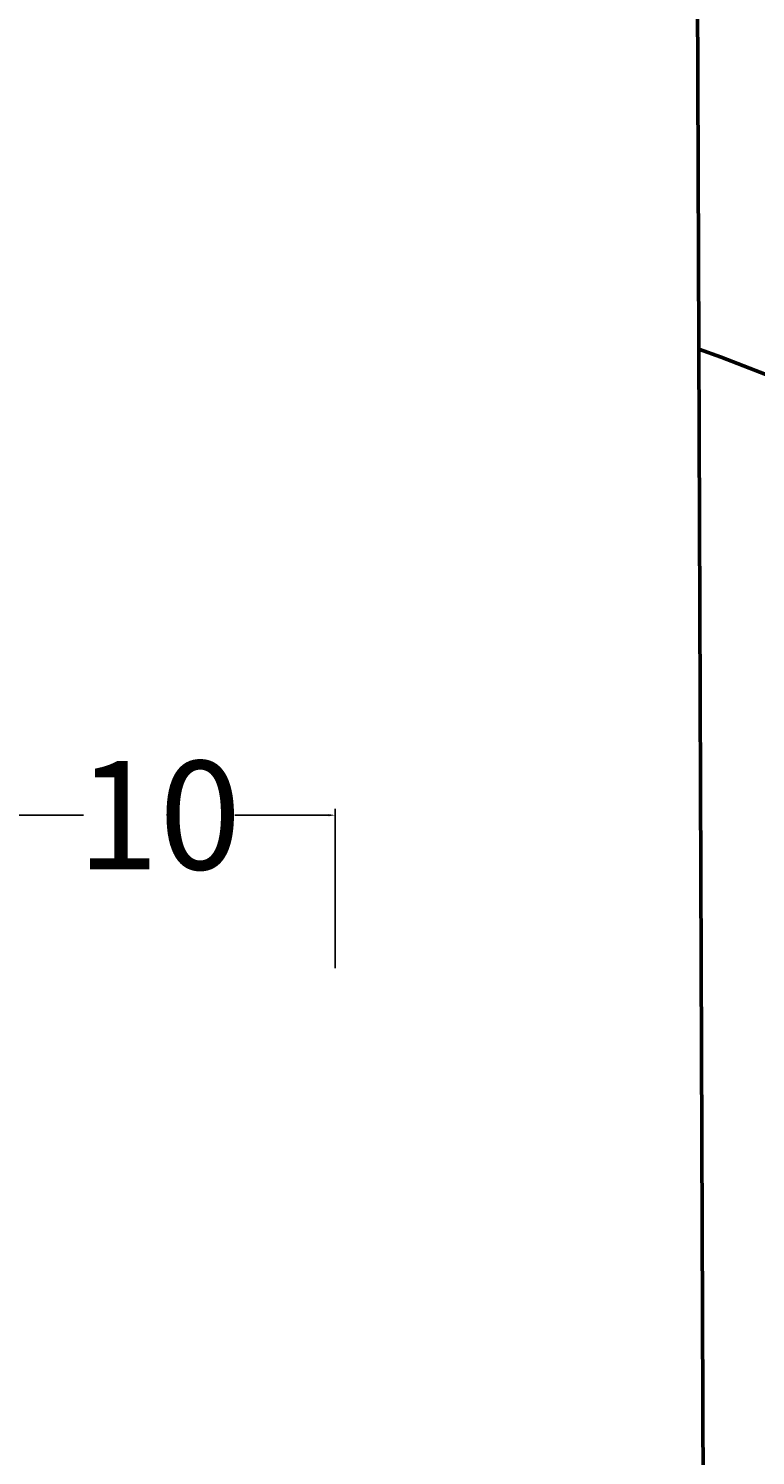
# Model space of a CAD drawing. Units: millimetres. Extents: x -53 to 92, y -147 to 37.
# Tile 13 of 16: x 20 to 40, y -30 to 9. Entities that reach past the tile are written whole.
import ezdxf

# ---------------------------------------------------------------- set-up
doc = ezdxf.new("R2010")
doc.units = ezdxf.units.MM
doc.header["$MEASUREMENT"] = 0
doc.layers.add('M-DIMS', color=2, linetype='Continuous', lineweight=25)
doc.layers.add('M-OUTL', color=7, linetype='Continuous', lineweight=50)
doc.styles.get("Standard").update_dxf_attribs({"font": 'arial.ttf'})
doc.dimstyles.get("Standard").update_dxf_attribs({"dimtxt": 0.18, "dimasz": 0.18, "dimexe": 0.18, "dimexo": 0.0625, "dimgap": 0.09, "dimtad": 0, "dimtih": 1, "dimtoh": 1, "dimdec": 4, "dimzin": 0, "dimdsep": 46, "dimtxsty": 'Standard', "dimcen": 0.09, "dimadec": 0, "dimazin": 0, "dimtfac": 1, "dimtdec": 4, "dimtofl": 0, "dimtmove": 0, "dimatfit": 3, "dimfxl": 1, "dimtolj": 1, "dimtzin": 0, "dimarcsym": 0})

# ---------------------------------------------------------------- blocks, each defined once
blk = doc.blocks.new('*D5')
at = {"layer": 'Defpoints', "color": 0, "transparency": 16777216}
for p in [(28.602, 35.845), (28.602, 15.91), (9.265, -3.88)]:
    blk.add_point(p, dxfattribs=at)
at = {"layer": 'M-DIMS', "color": 0, "lineweight": -2, "transparency": 16777216}
for p, q in [((9.265, -3.817), (9.265, 36.025)), ((28.602, 15.973), (28.602, 36.025)), ((9.445, 35.845), (16.674, 35.845)), ((28.422, 35.845), (21.192, 35.845))]:
    blk.add_line(p, q, dxfattribs=at)
at = {"layer": 'M-DIMS', "color": 0, "transparency": 16777216}
for points in [[(9.445, 35.875), (9.445, 35.815), (9.265, 35.845)], [(28.422, 35.875), (28.422, 35.815), (28.602, 35.845)]]:
    blk.add_solid(points, dxfattribs=at)
at = {"layer": 'M-DIMS', "color": 0, "transparency": 16777216, "insert": (18.933, 35.845), "char_height": 0.18, "attachment_point": 5}
blk.add_mtext('\\A1;{\\H16.66667x;20}', dxfattribs=at)
blk = doc.blocks.new('*D6')
at = {"layer": 'Defpoints', "color": 0, "transparency": 16777216}
for p in [(-26.95, 15.91), (28.602, 15.91), (9.355, -3.79)]:
    blk.add_point(p, dxfattribs=at)
at = {"layer": 'M-DIMS', "color": 0, "lineweight": -2, "transparency": 16777216}
for p, q in [((28.539, 15.91), (-27.13, 15.91)), ((-26.95, 15.73), (-26.95, 7.682)), ((-26.95, -3.61), (-26.95, 4.438)), ((9.292, -3.79), (-27.13, -3.79))]:
    blk.add_line(p, q, dxfattribs=at)
at = {"layer": 'M-DIMS', "color": 0, "transparency": 16777216}
for points in [[(-26.98, 15.73), (-26.92, 15.73), (-26.95, 15.91)], [(-26.98, -3.61), (-26.92, -3.61), (-26.95, -3.79)]]:
    blk.add_solid(points, dxfattribs=at)
at = {"layer": 'M-DIMS', "color": 0, "transparency": 16777216, "insert": (-26.95, 6.06), "char_height": 0.18, "attachment_point": 5}
blk.add_mtext('\\A1;{\\H16.66667x;20}', dxfattribs=at)
blk = doc.blocks.new('*D10')
at = {"layer": 'Defpoints', "color": 0, "transparency": 16777216}
for p in [(64.593, -18.184), (-26.68, -89.776)]:
    blk.add_point(p, dxfattribs=at)
at = {"layer": 'M-DIMS', "color": 0, "lineweight": -2, "transparency": 16777216}
for p, q in [((77.384, -8.151), (64.734, -18.073)), ((77.564, -8.151), (77.384, -8.151)), ((18.866, -53.98), (19.046, -53.98)), ((18.956, -54.07), (18.956, -53.89))]:
    blk.add_line(p, q, dxfattribs=at)
at = {"layer": 'M-DIMS', "color": 0, "transparency": 16777216}
blk.add_solid([(64.716, -18.05), (64.753, -18.097), (64.593, -18.184)], dxfattribs=at)
at = {"layer": 'M-DIMS', "color": 0, "transparency": 16777216, "insert": (82.599, -8.151), "char_height": 0.18, "attachment_point": 5}
blk.add_mtext('\\A1;{\\H16.66667x;%%C116}', dxfattribs=at)
blk = doc.blocks.new('*D14')
at = {"layer": 'Defpoints', "color": 0, "transparency": 16777216}
for p in [(28.692, -12.346), (18.956, -15.584), (28.692, -16.641)]:
    blk.add_point(p, dxfattribs=at)
at = {"layer": 'M-DIMS', "color": 0, "lineweight": -2, "transparency": 16777216}
for p, q in [((18.956, -15.521), (18.956, -12.166)), ((28.692, -16.578), (28.692, -12.166)), ((19.136, -12.346), (21.732, -12.346)), ((28.512, -12.346), (25.917, -12.346))]:
    blk.add_line(p, q, dxfattribs=at)
at = {"layer": 'M-DIMS', "color": 0, "transparency": 16777216}
for points in [[(19.136, -12.316), (19.136, -12.376), (18.956, -12.346)], [(28.512, -12.316), (28.512, -12.376), (28.692, -12.346)]]:
    blk.add_solid(points, dxfattribs=at)
at = {"layer": 'M-DIMS', "color": 0, "transparency": 16777216, "insert": (23.824, -12.346), "char_height": 0.18, "attachment_point": 5}
blk.add_mtext('\\A1;{\\H16.66667x;10}', dxfattribs=at)
blk = doc.blocks.new('*D17')
at = {"layer": 'Defpoints', "color": 0, "transparency": 16777216}
for p in [(-46.81, 25.909), (28.564, 25.909), (18.165, -111.975)]:
    blk.add_point(p, dxfattribs=at)
at = {"layer": 'M-DIMS', "color": 0, "lineweight": -2, "transparency": 16777216}
for p, q in [((28.502, 25.909), (-46.99, 25.909)), ((-46.81, 25.729), (-46.81, -42.851)), ((-46.81, -111.795), (-46.81, -43.215)), ((18.102, -111.975), (-46.99, -111.975))]:
    blk.add_line(p, q, dxfattribs=at)
at = {"layer": 'M-DIMS', "color": 0, "transparency": 16777216}
for points in [[(-46.84, 25.729), (-46.78, 25.729), (-46.81, 25.909)], [(-46.84, -111.795), (-46.78, -111.795), (-46.81, -111.975)]]:
    blk.add_solid(points, dxfattribs=at)
at = {"layer": 'M-DIMS', "color": 0, "transparency": 16777216, "insert": (-46.81, -43.033), "char_height": 0.18, "attachment_point": 5}
blk.add_mtext('\\A1;137.88', dxfattribs=at)

msp = doc.modelspace()

# ---------------------------------------------------------------- linework, layer by layer
at = {"layer": 'M-OUTL'}
msp.add_line((38.69188, 15.90293), (38.97226, -58.39443), dxfattribs=at)
msp.add_arc((18.95638, -53.98007), 58, 108.3895553, 70.0459142, dxfattribs=at)

# ---------------------------------------------------------------- dimensions: what is measured, and where the dimension line sits
at = {"layer": 'M-DIMS'}
for base, p1, p2, text, picture, middle in [((28.60189, 35.84496), (9.26461, -3.87977), (28.60189, 15.91006), '{\\H16.66667x;20}', '*D5', (18.93325, 35.84496)), ((28.69189, -12.34633), (18.95638, -15.58399), (28.69189, -16.64088), '{\\H16.66667x;10}', '*D14', (23.82413, -12.34633))]:
    dim = msp.add_linear_dim(base=base, p1=p1, p2=p2, text=text, dimstyle='Standard', override={"dimclrd": 0, "dimclre": 0, "dimclrt": 0}, dxfattribs=at)
    dim.commit()
    dim.dimension.update_dxf_attribs({"geometry": picture, "text_midpoint": middle})
dim = msp.add_linear_dim(base=(-46.8103, 25.90924), p1=(18.16452, -111.97467), p2=(28.56407, 25.90924), angle=90, dimstyle='Standard', override={"dimdec": 2, "dimlfac": 1, "dimrnd": 0, "dimzin": 0, "dimdsep": 46, "dimlunit": 2}, dxfattribs=at)
dim.commit()
dim.dimension.update_dxf_attribs({"geometry": '*D17', "text_midpoint": (-46.8103, -43.03271)})
dim = msp.add_linear_dim(base=(-26.95014, 15.91006), p1=(9.35461, -3.78977), p2=(28.60189, 15.91006), angle=90, text='{\\H16.66667x;20}', dimstyle='Standard', override={"dimclrd": 0, "dimclre": 0, "dimclrt": 0}, dxfattribs=at)
dim.commit()
dim.dimension.update_dxf_attribs({"geometry": '*D6', "text_midpoint": (-26.95014, 6.06014)})
dim = msp.add_diameter_dim_2p(p1=(-26.67986, -89.77579), p2=(64.59262, -18.18435), text='{\\H16.66667x;%%C116}', dimstyle='Standard', override={"dimclrd": 0, "dimclre": 0, "dimclrt": 0}, dxfattribs=at)
dim.commit()
dim.dimension.update_dxf_attribs({"geometry": '*D10', "text_midpoint": (82.59889, -8.15132), "dimtype": 163})

doc.saveas('drawing.dxf')
